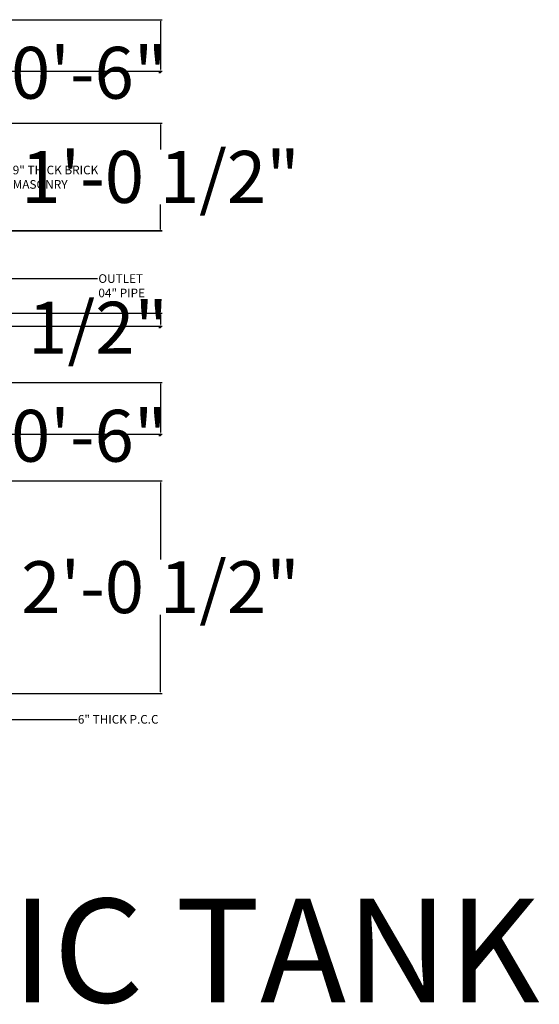
# Model space of a CAD drawing. Units: inches. Extents: x -34 to 285, y -151 to 155.
# Tile 9 of 10: x 225 to 285, y -151 to -37. Entities that reach past the tile are written whole.
import ezdxf
from ezdxf import colors
from ezdxf.entities.mleader import LeaderData, LeaderLine
from ezdxf.math import Vec2, Vec3

# ---------------------------------------------------------------- set-up
doc = ezdxf.new("R2010")
doc.units = ezdxf.units.IN
doc.header["$MEASUREMENT"] = 0
doc.layers.add('A-ANNO-DIMS', color=2, linetype='Continuous', lineweight=18)
doc.layers.add('A-ANNO-TEXT', color=7, linetype='Continuous', lineweight=25)
doc.styles.get("Standard").update_dxf_attribs({"font": 'arial.ttf'})
doc.dimstyles.get("Standard").update_dxf_attribs({"dimtxt": 6, "dimasz": 0.18, "dimexe": 0.18, "dimexo": 0.0625, "dimgap": 0.09, "dimtad": 0, "dimtih": 1, "dimtoh": 1, "dimzin": 0, "dimdsep": 46, "dimlunit": 3, "dimtxsty": 'Standard', "dimcen": 0.09, "dimadec": 0, "dimazin": 0, "dimtfac": 1, "dimtofl": 0, "dimtmove": 0, "dimatfit": 3, "dimfxl": 1, "dimtolj": 1, "dimtzin": 0, "dimarcsym": 0})

# ---------------------------------------------------------------- blocks, each defined once
blk = doc.blocks.new('*D56')
at = {"layer": 'A-ANNO-DIMS', "color": 0, "lineweight": -2, "transparency": 16777216}
for p, q in [((46.49, -37.01), (241.64, -37.01)), ((241.46, -37.19), (241.46, -42.79)), ((46.49, -42.97), (241.64, -42.97)), ((241.46, -43.15), (241.28, -43.15)), ((241.46, -42.97), (241.46, -43.15))]:
    blk.add_line(p, q, dxfattribs=at)
at = {"layer": 'A-ANNO-DIMS', "color": 0, "transparency": 16777216}
for points in [[(241.43, -37.19), (241.49, -37.19), (241.46, -37.01)], [(241.43, -42.79), (241.49, -42.79), (241.46, -42.97)]]:
    blk.add_solid(points, dxfattribs=at)
at = {"layer": 'Defpoints', "color": 0, "transparency": 16777216}
for p in [(46.43, -37.01), (46.43, -42.97), (241.46, -42.97)]:
    blk.add_point(p, dxfattribs=at)
at = {"layer": 'A-ANNO-DIMS', "color": 0, "transparency": 16777216, "insert": (233.21, -43.15), "char_height": 6, "attachment_point": 5}
blk.add_mtext('\\A1;0\'-6"', dxfattribs=at)
blk = doc.blocks.new('*D59')
at = {"layer": 'A-ANNO-DIMS', "color": 0, "lineweight": -2, "transparency": 16777216}
for p, q in [((83.15, -48.97), (241.64, -48.97)), ((241.46, -49.15), (241.46, -52)), ((241.46, -61.23), (241.46, -58.38)), ((89.01, -61.41), (241.64, -61.41))]:
    blk.add_line(p, q, dxfattribs=at)
at = {"layer": 'A-ANNO-DIMS', "color": 0, "transparency": 16777216}
for points in [[(241.43, -49.15), (241.49, -49.15), (241.46, -48.97)], [(241.43, -61.23), (241.49, -61.23), (241.46, -61.41)]]:
    blk.add_solid(points, dxfattribs=at)
at = {"layer": 'Defpoints', "color": 0, "transparency": 16777216}
for p in [(83.09, -48.97), (88.95, -61.41), (241.46, -61.41)]:
    blk.add_point(p, dxfattribs=at)
at = {"layer": 'A-ANNO-DIMS', "color": 0, "transparency": 16777216, "insert": (241.46, -55.19), "char_height": 6, "attachment_point": 5}
blk.add_mtext('\\A1;1\'-0 1/2"', dxfattribs=at)
blk = doc.blocks.new('*D62')
at = {"layer": 'A-ANNO-DIMS', "color": 0, "lineweight": -2, "transparency": 16777216}
for p, q in [((155.22, -48.97), (241.64, -48.97)), ((241.46, -49.15), (241.46, -52.02)), ((241.46, -61.27), (241.46, -58.4)), ((153.78, -61.45), (241.64, -61.45))]:
    blk.add_line(p, q, dxfattribs=at)
at = {"layer": 'A-ANNO-DIMS', "color": 0, "transparency": 16777216}
for points in [[(241.43, -49.15), (241.49, -49.15), (241.46, -48.97)], [(241.43, -61.27), (241.49, -61.27), (241.46, -61.45)]]:
    blk.add_solid(points, dxfattribs=at)
at = {"layer": 'Defpoints', "color": 0, "transparency": 16777216}
for p in [(155.16, -48.97), (153.71, -61.45), (241.46, -61.45)]:
    blk.add_point(p, dxfattribs=at)
at = {"layer": 'A-ANNO-DIMS', "color": 0, "transparency": 16777216, "insert": (241.46, -55.21), "char_height": 6, "attachment_point": 5}
blk.add_mtext('\\A1;1\'-0 1/2"', dxfattribs=at)
blk = doc.blocks.new('*D65')
at = {"layer": 'A-ANNO-DIMS', "color": 0, "lineweight": -2, "transparency": 16777216}
for p, q in [((130.16, -90.37), (241.64, -90.37)), ((241.46, -90.55), (241.46, -99.48)), ((241.46, -114.79), (241.46, -105.86)), ((139.91, -114.97), (241.64, -114.97))]:
    blk.add_line(p, q, dxfattribs=at)
at = {"layer": 'A-ANNO-DIMS', "color": 0, "transparency": 16777216}
for points in [[(241.43, -90.55), (241.49, -90.55), (241.46, -90.37)], [(241.43, -114.79), (241.49, -114.79), (241.46, -114.97)]]:
    blk.add_solid(points, dxfattribs=at)
at = {"layer": 'Defpoints', "color": 0, "transparency": 16777216}
for p in [(130.1, -90.37), (139.85, -114.97), (241.46, -114.97)]:
    blk.add_point(p, dxfattribs=at)
at = {"layer": 'A-ANNO-DIMS', "color": 0, "transparency": 16777216, "insert": (241.46, -102.67), "char_height": 6, "attachment_point": 5}
blk.add_mtext('\\A1;2\'-0 1/2"', dxfattribs=at)
blk = doc.blocks.new('*D66')
at = {"layer": 'A-ANNO-DIMS', "color": 0, "lineweight": -2, "transparency": 16777216}
for p, q in [((157.91, -78.97), (241.64, -78.97)), ((241.46, -79.15), (241.46, -84.79)), ((157.91, -84.97), (241.64, -84.97)), ((241.46, -85.15), (241.28, -85.15)), ((241.46, -84.97), (241.46, -85.15))]:
    blk.add_line(p, q, dxfattribs=at)
at = {"layer": 'A-ANNO-DIMS', "color": 0, "transparency": 16777216}
for points in [[(241.43, -79.15), (241.49, -79.15), (241.46, -78.97)], [(241.43, -84.79), (241.49, -84.79), (241.46, -84.97)]]:
    blk.add_solid(points, dxfattribs=at)
at = {"layer": 'Defpoints', "color": 0, "transparency": 16777216}
for p in [(157.85, -78.97), (157.85, -84.97), (241.46, -84.97)]:
    blk.add_point(p, dxfattribs=at)
at = {"layer": 'A-ANNO-DIMS', "color": 0, "transparency": 16777216, "insert": (233.21, -85.15), "char_height": 6, "attachment_point": 5}
blk.add_mtext('\\A1;0\'-6"', dxfattribs=at)
blk = doc.blocks.new('*D78')
at = {"layer": 'A-ANNO-DIMS', "color": 0, "lineweight": -2, "transparency": 16777216}
for p, q in [((96.29, -70.95), (241.64, -70.95)), ((241.46, -71.13), (241.46, -72.29)), ((96.29, -72.47), (241.64, -72.47)), ((241.46, -72.65), (241.28, -72.65)), ((241.46, -72.47), (241.46, -72.65))]:
    blk.add_line(p, q, dxfattribs=at)
at = {"layer": 'A-ANNO-DIMS', "color": 0, "transparency": 16777216}
for points in [[(241.43, -71.13), (241.49, -71.13), (241.46, -70.95)], [(241.43, -72.29), (241.49, -72.29), (241.46, -72.47)]]:
    blk.add_solid(points, dxfattribs=at)
at = {"layer": 'Defpoints', "color": 0, "transparency": 16777216}
for p in [(96.23, -70.95), (96.23, -72.47), (241.46, -72.47)]:
    blk.add_point(p, dxfattribs=at)
at = {"layer": 'A-ANNO-DIMS', "color": 0, "transparency": 16777216, "insert": (226.22, -72.65), "char_height": 6, "attachment_point": 5}
blk.add_mtext('\\A1;0\'-1 1/2"', dxfattribs=at)

msp = doc.modelspace()

# ---------------------------------------------------------------- texts
at = {"layer": 'A-ANNO-TEXT', "insert": (-34.52, -138.72), "char_height": 12, "attachment_point": 1}
msp.add_mtext_dynamic_manual_height_columns('SECTIONAL ELEVATION OF A SEPTIC TANK ', width=509.35271, gutter_width=1, heights=[0], dxfattribs=at)

# ---------------------------------------------------------------- dimensions: what is measured, and where the dimension line sits
at = {"layer": 'A-ANNO-DIMS'}
for base, p1, p2, picture, middle in [((241.457, -42.969), (46.43, -37.008), (46.43, -42.969), '*D56', (233.213, -43.149)), ((241.457, -61.415), (83.086, -48.969), (88.947, -61.415), '*D59', (241.457, -55.192)), ((241.457, -61.451), (155.156, -48.969), (153.715, -61.451), '*D62', (241.457, -55.21)), ((241.457, -72.47), (96.231, -70.947), (96.231, -72.47), '*D78', (226.222, -72.65)), ((241.457, -84.969), (157.846, -78.969), (157.846, -84.969), '*D66', (233.213, -85.149)), ((241.457, -114.969), (130.096, -90.369), (139.846, -114.969), '*D65', (241.457, -102.669))]:
    dim = msp.add_linear_dim(base=base, p1=p1, p2=p2, angle=90, dimstyle='Standard', override={"dimdec": 1, "dimlfac": 1, "dimrnd": 0, "dimzin": 1, "dimdsep": 46, "dimlunit": 4, "dimfrac": 2}, dxfattribs=at)
    dim.commit()
    dim.dimension.update_dxf_attribs({"geometry": picture, "text_midpoint": middle})

# ---------------------------------------------------------------- leaders
at = {"layer": 'A-ANNO-TEXT'}
ml = msp.add_multileader_mtext('Standard', dxfattribs=at)
ml.set_content('9" THICK BRICK \\PMASONRY ', color=(248, 215, 49))
ml.set_leader_properties()
ml.build(insert=Vec2(0, 0))
ml.multileader.update_dxf_attribs({"dogleg_length": 4.22, "arrow_head_size": 3})
ctx = ml.context
ctx.base_point, ctx.char_height, ctx.arrow_head_size, ctx.landing_gap_size, ctx.plane_origin = Vec3(224.277, -54.411), 1, 3, 0.09, Vec3(205.846, -54.411)
notes = []
notes.append((ctx, [(0, (1, 1, 0), (220.057, -54.411), (1, 0), 4.22, [(0, [(205.846, -54.411)], 0, [])])]))
ctx.mtext.insert, ctx.mtext.flow_direction = Vec3(224.367, -53.902), 5
ml = msp.add_multileader_mtext('Standard', dxfattribs=at)
ml.set_content('OUTLET\\P04" PIPE', color=(248, 215, 49))
ml.set_leader_properties()
ml.build(insert=Vec2(0, 0))
ml.multileader.update_dxf_attribs({"dogleg_length": 4.22, "arrow_head_size": 3})
ctx = ml.context
ctx.base_point, ctx.char_height, ctx.arrow_head_size, ctx.landing_gap_size, ctx.plane_origin = Vec3(234.182, -66.969), 1, 3, 0.09, Vec3(214.207, -66.969)
notes.append((ctx, [(0, (1, 1, 0), (229.962, -66.969), (1, 0), 4.22, [(0, [(214.207, -66.969)], 0, [])])]))
ctx.mtext.insert, ctx.mtext.flow_direction = Vec3(234.272, -66.46), 5
ml = msp.add_multileader_mtext('Standard', dxfattribs=at)
ml.set_content('6" THICK P.C.C ', color=(248, 215, 49))
ml.set_leader_properties()
ml.build(insert=Vec2(0, 0))
ml.multileader.update_dxf_attribs({"dogleg_length": 4.22, "arrow_head_size": 3})
ctx = ml.context
ctx.base_point, ctx.char_height, ctx.arrow_head_size, ctx.landing_gap_size, ctx.plane_origin = Vec3(231.808, -117.969), 1, 3, 0.09, Vec3(214.846, -117.969)
notes.append((ctx, [(0, (1, 1, 0), (227.588, -117.969), (1, 0), 4.22, [(0, [(214.846, -117.969)], 0, [])])]))
ctx.mtext.insert, ctx.mtext.flow_direction = Vec3(231.898, -117.46), 5
for ctx, leaders in notes:
    for number, flags, end, landing, length, lines in leaders:
        leader = LeaderData()
        leader.index, (leader.has_last_leader_line, leader.has_dogleg_vector, leader.attachment_direction) = number, flags
        leader.last_leader_point, leader.dogleg_vector, leader.dogleg_length = Vec3(end), Vec3(landing), length
        for number, points, colour, breaks in lines:
            line = LeaderLine()
            line.index, line.vertices, line.color, line.breaks = number, Vec3.list(points), colors.encode_raw_color(colour), breaks
            leader.lines.append(line)
        ctx.leaders.append(leader)

doc.saveas('drawing.dxf')
